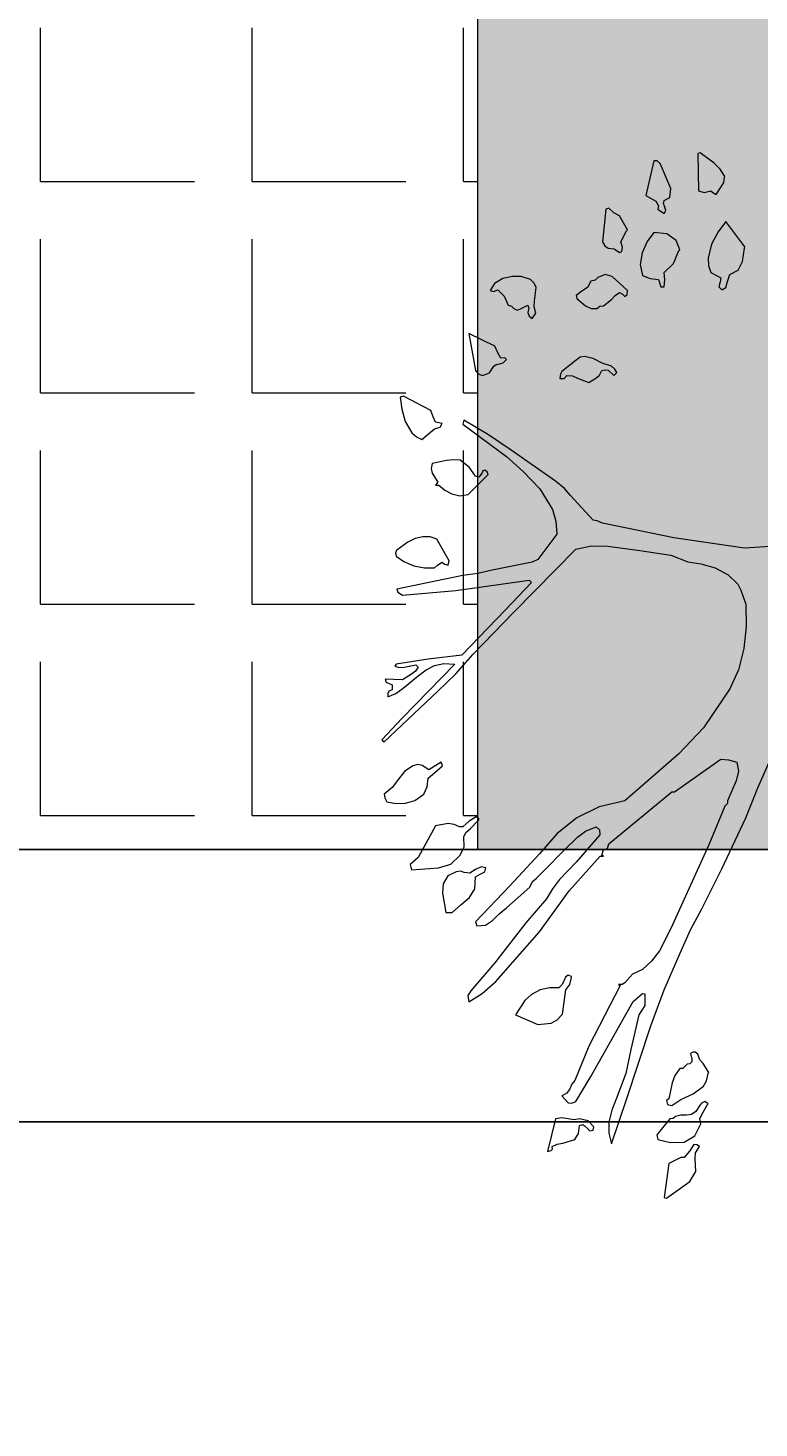
# Model space of a CAD drawing. Units: inches. Extents: x 84 to 1044, y -280 to 906.
# Tile 16 of 105: x 635 to 659, y -132 to -86. Entities that reach past the tile are written whole.
import ezdxf

# ---------------------------------------------------------------- set-up
doc = ezdxf.new("R2010")
doc.units = ezdxf.units.IN
for name, color, linetype, lineweight in [('A-ANNO-DIMS', 2, 'Continuous', 18), ('C-PROP', 7, 'Continuous', 25), ('L-HRDS', 32, 'Continuous', 18), ('L-PLNT', 114, 'Continuous', 15)]:
    doc.layers.add(name, color=color, linetype=linetype, lineweight=lineweight)
doc.layers.add('L-HRDS-PATT', color=23, linetype='Continuous', lineweight=9, true_color=0xc2877b)
doc.layers.add('L-PLNT-PATT', color=9, linetype='Continuous', lineweight=9, true_color=0xafd9aa)
doc.styles.get("Standard").update_dxf_attribs({"font": 'arial.ttf'})
doc.dimstyles.get("Standard").update_dxf_attribs({"dimtxt": 0.18, "dimasz": 0.18, "dimexe": 0.18, "dimexo": 0.0625, "dimgap": 0.09, "dimtad": 0, "dimtih": 1, "dimtoh": 1, "dimdec": 4, "dimzin": 0, "dimdsep": 46, "dimtxsty": 'Standard', "dimcen": 0.09, "dimadec": 0, "dimazin": 0, "dimtfac": 1, "dimtdec": 4, "dimtofl": 0, "dimtmove": 0, "dimatfit": 3, "dimfxl": 1, "dimtolj": 1, "dimtzin": 0, "dimarcsym": 0})

# ---------------------------------------------------------------- blocks, each defined once
blk = doc.blocks.new('A$C37E508DF')
for p, q in [((0.9686, 1.4334), (0.9875, 1.4476)), ((0.9875, 1.4476), (0.9905, 1.4467)), ((0.9905, 1.4467), (0.9896, 1.3966)), ((0.9605, 1.4257), (0.9686, 1.4334)), ((1.0269, 1.3996), (1.0411, 1.433)), ((1.0411, 1.433), (1.045, 1.4365)), ((1.045, 1.4365), (1.0497, 1.4369)), ((1.0497, 1.4369), (1.0604, 1.3901)), ((0.9545, 1.4159), (0.9605, 1.4257)), ((0.9549, 1.4146), (0.9545, 1.4159)), ((0.9558, 1.4077), (0.9549, 1.4146)), ((0.9592, 1.4017), (0.9558, 1.4077)), ((0.966, 1.3914), (0.9592, 1.4017)), ((0.9703, 1.3944), (0.966, 1.3914)), ((0.9733, 1.3966), (0.9703, 1.3944)), ((0.9819, 1.3944), (0.9733, 1.3966)), ((0.9896, 1.3966), (0.9819, 1.3944)), ((1.0282, 1.3876), (1.0269, 1.3996)), ((1.0604, 1.3901), (1.0471, 1.3824)), ((1.0359, 1.3833), (1.0282, 1.3876)), ((1.0334, 1.37), (1.0351, 1.376)), ((1.0351, 1.376), (1.0368, 1.3794)), ((1.0368, 1.3794), (1.0359, 1.3833)), ((1.0441, 1.3717), (1.0359, 1.3661)), ((1.0471, 1.3824), (1.0432, 1.3764)), ((1.0432, 1.3764), (1.0441, 1.3717)), ((1.1033, 1.367), (1.1097, 1.373)), ((1.1097, 1.373), (1.114, 1.3717)), ((1.114, 1.3717), (1.1183, 1.328)), ((0.9274, 1.3215), (0.9532, 1.3554)), ((0.9532, 1.3554), (0.9635, 1.3413)), ((1.0359, 1.3661), (1.0334, 1.37)), ((1.0848, 1.3443), (1.0955, 1.3631)), ((1.0955, 1.3631), (1.1033, 1.367)), ((0.9635, 1.3413), (0.9721, 1.325)), ((1.0197, 1.3297), (1.0321, 1.3387)), ((1.0321, 1.3387), (1.0497, 1.3404)), ((1.0497, 1.3404), (1.0587, 1.3284)), ((1.0861, 1.343), (1.0848, 1.3443)), ((1.0938, 1.328), (1.0861, 1.343)), ((0.9279, 1.3194), (0.9274, 1.3215)), ((0.9305, 1.3018), (0.9279, 1.3194)), ((0.9721, 1.325), (0.9768, 1.3061)), ((1.0149, 1.3172), (1.0171, 1.3232)), ((1.0162, 1.3164), (1.0149, 1.3172)), ((1.0231, 1.2988), (1.0162, 1.3164)), ((1.0171, 1.3232), (1.0197, 1.3297)), ((1.0587, 1.3284), (1.0651, 1.3134)), ((1.0917, 1.3207), (1.0938, 1.328)), ((1.0925, 1.3151), (1.0917, 1.3207)), ((1.0955, 1.3138), (1.0925, 1.3151)), ((1.1028, 1.3185), (1.0955, 1.3138)), ((1.111, 1.3194), (1.1028, 1.3185)), ((1.1153, 1.3228), (1.111, 1.3194)), ((1.1183, 1.328), (1.1153, 1.3228)), ((0.9365, 1.2902), (0.9305, 1.3018)), ((0.9763, 1.2962), (0.9733, 1.2868)), ((0.9768, 1.3061), (0.9763, 1.2962)), ((1.0359, 1.2868), (1.0231, 1.2988)), ((1.0677, 1.2975), (1.0647, 1.2829)), ((1.0651, 1.3134), (1.0677, 1.2975)), ((0.9476, 1.2842), (0.9365, 1.2902)), ((0.951, 1.2748), (0.9476, 1.2842)), ((0.9733, 1.2868), (0.9596, 1.2799)), ((0.9596, 1.2799), (0.9605, 1.2744)), ((1.0347, 1.2769), (1.0359, 1.2868)), ((1.0359, 1.2679), (1.0347, 1.2769)), ((1.0432, 1.2774), (1.0402, 1.2679)), ((1.0544, 1.2791), (1.0432, 1.2774)), ((1.0647, 1.2829), (1.0544, 1.2791)), ((1.0848, 1.2628), (1.1054, 1.2817)), ((1.1054, 1.2817), (1.1148, 1.2842)), ((1.1148, 1.2842), (1.1247, 1.2804)), ((1.1247, 1.2804), (1.1281, 1.2765)), ((1.21, 1.2726), (1.2147, 1.2774)), ((1.2147, 1.2774), (1.2276, 1.2817)), ((1.2276, 1.2817), (1.2392, 1.2817)), ((1.2392, 1.2817), (1.2521, 1.2787)), ((1.2521, 1.2787), (1.2632, 1.2722)), ((0.9532, 1.2666), (0.951, 1.2748)), ((0.9583, 1.2636), (0.9532, 1.2666)), ((0.9626, 1.2679), (0.9583, 1.2636)), ((0.9605, 1.2744), (0.9626, 1.2679)), ((1.0402, 1.2679), (1.0359, 1.2679)), ((1.0852, 1.2576), (1.0848, 1.2628)), ((1.0921, 1.2585), (1.0883, 1.2546)), ((1.0955, 1.2602), (1.0921, 1.2585)), ((1.1015, 1.2559), (1.0955, 1.2602)), ((1.1281, 1.2765), (1.1341, 1.2752)), ((1.1341, 1.2752), (1.1384, 1.2666)), ((1.1384, 1.2666), (1.1461, 1.2619)), ((1.1461, 1.2619), (1.1539, 1.2559)), ((1.2075, 1.2666), (1.21, 1.2726)), ((1.2096, 1.2491), (1.2075, 1.2666)), ((1.2585, 1.2636), (1.2503, 1.2551)), ((1.2645, 1.2615), (1.2585, 1.2636)), ((1.2632, 1.2722), (1.2692, 1.2628)), ((1.2692, 1.2628), (1.2645, 1.2615)), ((1.0883, 1.2546), (1.0852, 1.2576)), ((1.1063, 1.2508), (1.1015, 1.2559)), ((1.117, 1.2422), (1.1063, 1.2508)), ((1.1221, 1.2418), (1.117, 1.2422)), ((1.126, 1.2388), (1.1221, 1.2418)), ((1.141, 1.2422), (1.1337, 1.2388)), ((1.1526, 1.2521), (1.141, 1.2422)), ((1.1539, 1.2559), (1.1526, 1.2521)), ((1.2079, 1.2323), (1.21, 1.2409)), ((1.21, 1.2409), (1.2096, 1.2491)), ((1.2186, 1.2431), (1.2173, 1.2392)), ((1.2285, 1.2383), (1.2186, 1.2431)), ((1.2405, 1.2418), (1.2371, 1.2388)), ((1.2448, 1.2431), (1.2405, 1.2418)), ((1.2503, 1.2551), (1.2448, 1.2431)), ((1.1337, 1.2388), (1.126, 1.2388)), ((1.2126, 1.2251), (1.2079, 1.2323)), ((1.2169, 1.2285), (1.2126, 1.2251)), ((1.2186, 1.2332), (1.2169, 1.2285)), ((1.2173, 1.2392), (1.2186, 1.2332)), ((1.2328, 1.2366), (1.2285, 1.2383)), ((1.2371, 1.2388), (1.2328, 1.2366)), ((1.2628, 1.1882), (1.2975, 1.2053)), ((1.2975, 1.2053), (1.2885, 1.1556)), ((1.2589, 1.1792), (1.2628, 1.1882)), ((1.1063, 1.1612), (1.1187, 1.1655)), ((1.1187, 1.1655), (1.1307, 1.1714)), ((1.1307, 1.1714), (1.1423, 1.1744)), ((1.1423, 1.1744), (1.1483, 1.1732)), ((1.1483, 1.1732), (1.1539, 1.1693)), ((1.1539, 1.1693), (1.1727, 1.1543)), ((1.2469, 1.1702), (1.2495, 1.1723)), ((1.2478, 1.1693), (1.2469, 1.1702)), ((1.2516, 1.1659), (1.2478, 1.1693)), ((1.2495, 1.1723), (1.2546, 1.1719)), ((1.2563, 1.1646), (1.2516, 1.1659)), ((1.2546, 1.1719), (1.2589, 1.1792)), ((1.2611, 1.1637), (1.2563, 1.1646)), ((1.099, 1.153), (1.102, 1.1573)), ((1.1033, 1.1487), (1.099, 1.153)), ((1.102, 1.1573), (1.1063, 1.1612)), ((1.111, 1.156), (1.1033, 1.1487)), ((1.1153, 1.1564), (1.111, 1.156)), ((1.1191, 1.1556), (1.1153, 1.1564)), ((1.1226, 1.1492), (1.1191, 1.1556)), ((1.1273, 1.1453), (1.1226, 1.1492)), ((1.1586, 1.1483), (1.1517, 1.1453)), ((1.1663, 1.1487), (1.1586, 1.1483)), ((1.1697, 1.1449), (1.1663, 1.1487)), ((1.1727, 1.1543), (1.1749, 1.1504)), ((1.1749, 1.1504), (1.1757, 1.1449)), ((1.2641, 1.1612), (1.2611, 1.1637)), ((1.2701, 1.1522), (1.2641, 1.1612)), ((1.2791, 1.1487), (1.2701, 1.1522)), ((1.2851, 1.1509), (1.2791, 1.1487)), ((1.2885, 1.1556), (1.2851, 1.1509)), ((1.1367, 1.1393), (1.1273, 1.1453)), ((1.1517, 1.1453), (1.1367, 1.1393)), ((1.1757, 1.1449), (1.1697, 1.1449)), ((1.3485, 1.102), (1.385, 1.1209)), ((1.385, 1.1209), (1.3897, 1.1196)), ((1.3897, 1.1196), (1.3875, 1.1037)), ((1.3421, 1.0861), (1.3455, 1.0934)), ((1.3455, 1.0934), (1.3485, 1.102)), ((1.3875, 1.1037), (1.3828, 1.087)), ((1.3057, 1.0835), (1.2469, 1.0402)), ((1.2713, 1.0694), (1.3044, 1.0887)), ((1.3044, 1.0887), (1.3057, 1.0835)), ((1.3335, 1.0844), (1.3421, 1.0861)), ((1.3361, 1.0793), (1.3335, 1.0844)), ((1.3434, 1.0771), (1.3361, 1.0793)), ((1.349, 1.0728), (1.3434, 1.0771)), ((1.3605, 1.063), (1.349, 1.0728)), ((1.3738, 1.072), (1.3678, 1.0664)), ((1.3828, 1.087), (1.3738, 1.072)), ((1.2409, 1.0488), (1.2713, 1.0694)), ((1.3678, 1.0664), (1.3605, 1.063)), ((1.1813, 1.0072), (1.2409, 1.0488)), ((1.2469, 1.0402), (1.2246, 1.0201)), ((1.2971, 1.0257), (1.3091, 1.0351)), ((1.3091, 1.0351), (1.3185, 1.0355)), ((1.3185, 1.0355), (1.3275, 1.0347)), ((1.3275, 1.0347), (1.3468, 1.0308)), ((1.2246, 1.0201), (1.2023, 0.9969)), ((1.2718, 1.0162), (1.2731, 1.0197)), ((1.2984, 0.9892), (1.2718, 1.0162)), ((1.2731, 1.0197), (1.2761, 1.0218)), ((1.2761, 1.0218), (1.2786, 1.0209)), ((1.2786, 1.0209), (1.2799, 1.0184)), ((1.2799, 1.0184), (1.2842, 1.0124)), ((1.2885, 1.0136), (1.2971, 1.0257)), ((1.3468, 1.018), (1.3391, 1.0059)), ((1.3468, 1.0308), (1.3481, 1.0239)), ((1.3481, 1.0239), (1.3468, 1.018)), ((1.1612, 0.9879), (1.1693, 0.9974)), ((1.1693, 0.9974), (1.1813, 1.0072)), ((1.2023, 0.9969), (1.1852, 0.9691)), ((1.2842, 1.0124), (1.2885, 1.0136)), ((1.3297, 0.9952), (1.3202, 0.9901)), ((1.3378, 1.0016), (1.3297, 0.9952)), ((1.3421, 1.0016), (1.3378, 1.0016)), ((1.3391, 1.0059), (1.3421, 1.0016)), ((1.1311, 0.9549), (1.1612, 0.9879)), ((1.3095, 0.9875), (1.2984, 0.9892)), ((1.3202, 0.9901), (1.3095, 0.9875)), ((1.1852, 0.9691), (1.1809, 0.9532)), ((1.0227, 0.9309), (1.1183, 0.9506)), ((1.1183, 0.9506), (1.1256, 0.954)), ((1.1256, 0.954), (1.1311, 0.9549)), ((1.1809, 0.9532), (1.1796, 0.936)), ((0.9279, 0.9172), (1.0227, 0.9309)), ((1.1333, 0.9202), (1.1114, 0.9198)), ((1.1543, 0.9159), (1.1333, 0.9202)), ((1.1796, 0.936), (1.2049, 0.9022)), ((1.3241, 0.9), (1.3404, 0.9292)), ((1.3404, 0.9292), (1.3494, 0.9322)), ((1.3494, 0.9322), (1.3592, 0.9326)), ((1.3592, 0.9326), (1.3695, 0.93)), ((1.3695, 0.93), (1.3794, 0.9253)), ((1.3794, 0.9253), (1.394, 0.9146)), ((0.8936, 0.9193), (0.9279, 0.9172)), ((1.0269, 0.9077), (1.0042, 0.8987)), ((1.0685, 0.9142), (1.0269, 0.9077)), ((1.1114, 0.9198), (1.0685, 0.9142)), ((1.2371, 0.8314), (1.1543, 0.9159)), ((1.2049, 0.9022), (1.2126, 0.8983)), ((1.3948, 0.9065), (1.3846, 0.8992)), ((1.394, 0.9146), (1.3957, 0.9112)), ((1.3957, 0.9112), (1.3948, 0.9065)), ((0.9673, 0.8906), (0.9498, 0.8816)), ((0.9866, 0.8962), (0.9673, 0.8906)), ((1.0042, 0.8987), (0.9866, 0.8962)), ((1.2126, 0.8983), (1.2662, 0.8876)), ((1.2662, 0.8876), (1.2855, 0.8833)), ((1.2855, 0.8833), (1.3057, 0.8807)), ((1.3254, 0.8944), (1.3241, 0.9)), ((1.3301, 0.8957), (1.3254, 0.8944)), ((1.3335, 0.8983), (1.3301, 0.8957)), ((1.3395, 0.8944), (1.3335, 0.8983)), ((1.3434, 0.8906), (1.3395, 0.8944)), ((1.3571, 0.8906), (1.3434, 0.8906)), ((1.3713, 0.8936), (1.3571, 0.8906)), ((1.3846, 0.8992), (1.3713, 0.8936)), ((0.9369, 0.8687), (0.933, 0.861)), ((0.9498, 0.8816), (0.9369, 0.8687)), ((1.2169, 0.8743), (1.2135, 0.8713)), ((1.2135, 0.8713), (1.2491, 0.834)), ((1.3151, 0.8606), (1.2169, 0.8743)), ((1.3057, 0.8807), (1.394, 0.8623)), ((0.9296, 0.852), (0.9262, 0.8421)), ((0.933, 0.861), (0.9296, 0.852)), ((1.3863, 0.8541), (1.3151, 0.8606)), ((1.3927, 0.8584), (1.3863, 0.8541)), ((1.394, 0.8623), (1.3927, 0.8584)), ((0.9262, 0.8421), (0.9257, 0.8121)), ((1.2919, 0.7752), (1.2371, 0.8314)), ((1.2491, 0.834), (1.3069, 0.7735)), ((0.9257, 0.8121), (0.9287, 0.7825)), ((0.9287, 0.7825), (0.936, 0.7542)), ((1.3151, 0.7487), (1.2919, 0.7752)), ((1.3069, 0.7735), (1.352, 0.7684)), ((0.936, 0.7542), (0.9476, 0.7285)), ((1.3309, 0.7624), (1.3164, 0.7615)), ((1.3164, 0.7615), (1.3871, 0.6891)), ((1.3434, 0.7598), (1.3309, 0.7624)), ((1.355, 0.7538), (1.3434, 0.7598)), ((1.352, 0.7684), (1.3948, 0.7615)), ((1.3653, 0.7461), (1.355, 0.7538)), ((1.3687, 0.7607), (1.3657, 0.7577)), ((1.3657, 0.7577), (1.3691, 0.7521)), ((1.3841, 0.7577), (1.3687, 0.7607)), ((1.3691, 0.7521), (1.3743, 0.7482)), ((1.3914, 0.7572), (1.3841, 0.7577)), ((1.397, 0.759), (1.3914, 0.7572)), ((1.3948, 0.7615), (1.397, 0.759)), ((1.3391, 0.7255), (1.3151, 0.7487)), ((1.3854, 0.7294), (1.3653, 0.7461)), ((1.3743, 0.7482), (1.3863, 0.7405)), ((1.3863, 0.7405), (1.4099, 0.7414)), ((1.4086, 0.7375), (1.4004, 0.7337)), ((1.4004, 0.7337), (1.4004, 0.7272)), ((1.4099, 0.7414), (1.4086, 0.7375)), ((0.9476, 0.7285), (0.9828, 0.6762)), ((1.4116, 0.6569), (1.3391, 0.7255)), ((1.3953, 0.7221), (1.3854, 0.7294)), ((1.4064, 0.7178), (1.3953, 0.7221)), ((1.4004, 0.7272), (1.4047, 0.7255)), ((1.4047, 0.7255), (1.406, 0.7221)), ((1.406, 0.7221), (1.4064, 0.7178)), ((0.9828, 0.6762), (1.0162, 0.6415)), ((1.3871, 0.6891), (1.4141, 0.6599)), ((1.4141, 0.6599), (1.4116, 0.6569)), ((1.0162, 0.6415), (1.0574, 0.605)), ((0.9103, 0.5956), (0.8932, 0.6342)), ((0.9382, 0.6303), (0.936, 0.6179)), ((0.9493, 0.6333), (0.9382, 0.6303)), ((0.9596, 0.6342), (0.9493, 0.6333)), ((1.0218, 0.5904), (0.9596, 0.6342)), ((1.3327, 0.6252), (1.3348, 0.6303)), ((1.343, 0.6162), (1.3327, 0.6252)), ((1.3348, 0.6303), (1.3511, 0.62)), ((1.3511, 0.62), (1.3601, 0.6256)), ((1.3601, 0.6256), (1.3661, 0.6269)), ((1.3661, 0.6269), (1.3725, 0.6252)), ((1.3725, 0.6252), (1.3837, 0.6175)), ((0.936, 0.6179), (0.939, 0.605)), ((0.939, 0.605), (0.9506, 0.5784)), ((1.0574, 0.605), (1.0883, 0.5784)), ((1.352, 0.6089), (1.343, 0.6162)), ((1.3533, 0.5969), (1.352, 0.6089)), ((1.3837, 0.6175), (1.3918, 0.6072)), ((1.3918, 0.6072), (1.4004, 0.5964)), ((0.9262, 0.5557), (0.9103, 0.5956)), ((1.0256, 0.5904), (1.0218, 0.5904)), ((1.1097, 0.5205), (1.0256, 0.5904)), ((1.358, 0.5874), (1.3533, 0.5969)), ((1.37, 0.5789), (1.358, 0.5874)), ((1.4004, 0.5964), (1.4111, 0.5874)), ((1.4103, 0.5823), (1.4077, 0.5771)), ((1.4111, 0.5874), (1.4103, 0.5823)), ((0.9506, 0.5784), (0.951, 0.5746)), ((0.951, 0.5746), (0.9545, 0.5711)), ((0.9545, 0.5711), (0.9759, 0.5193)), ((1.0883, 0.5784), (1.123, 0.5703)), ((1.123, 0.5703), (1.1526, 0.5557)), ((1.3824, 0.575), (1.37, 0.5789)), ((1.3953, 0.5746), (1.3824, 0.575)), ((1.4077, 0.5771), (1.3953, 0.5746)), ((0.9583, 0.4871), (0.9262, 0.5557)), ((1.1526, 0.5557), (1.1792, 0.5347)), ((1.2842, 0.554), (1.2855, 0.5557)), ((1.2842, 0.5527), (1.2842, 0.554)), ((1.2958, 0.5407), (1.2842, 0.5527)), ((1.2855, 0.5557), (1.2876, 0.557)), ((1.2876, 0.557), (1.2971, 0.551)), ((1.2971, 0.551), (1.3057, 0.5433)), ((1.3099, 0.5433), (1.3172, 0.5467)), ((1.3172, 0.5467), (1.3254, 0.548)), ((1.3254, 0.548), (1.3421, 0.5446)), ((1.3421, 0.5446), (1.3657, 0.5021)), ((1.1226, 0.5394), (1.1221, 0.5325)), ((1.1221, 0.5325), (1.1539, 0.4961)), ((1.1268, 0.5433), (1.1226, 0.5394)), ((1.141, 0.5377), (1.1268, 0.5433)), ((1.1521, 0.5296), (1.141, 0.5377)), ((1.1706, 0.5111), (1.1521, 0.5296)), ((1.1792, 0.5347), (1.2027, 0.5072)), ((1.3014, 0.536), (1.2958, 0.5407)), ((1.3044, 0.53), (1.3014, 0.536)), ((1.3039, 0.5167), (1.3044, 0.53)), ((1.3057, 0.5433), (1.3099, 0.5433)), ((0.9759, 0.5193), (1.0269, 0.4069)), ((1.1118, 0.5145), (1.1097, 0.5205)), ((1.117, 0.5124), (1.1118, 0.5145)), ((1.1191, 0.5055), (1.117, 0.5124)), ((1.1955, 0.4858), (1.1706, 0.5111)), ((1.2027, 0.5072), (1.2426, 0.4644)), ((1.3091, 0.5055), (1.3039, 0.5167)), ((1.117, 0.5042), (1.1191, 0.5055)), ((1.1217, 0.5042), (1.117, 0.5042)), ((1.1633, 0.4575), (1.1217, 0.5042)), ((1.1539, 0.4961), (1.1762, 0.4729)), ((1.2748, 0.4884), (1.2812, 0.4897)), ((1.2761, 0.4832), (1.2748, 0.4884)), ((1.2812, 0.4897), (1.2885, 0.4862)), ((1.3215, 0.4935), (1.3091, 0.5055)), ((1.3382, 0.4884), (1.3215, 0.4935)), ((1.3743, 0.4858), (1.3382, 0.4884)), ((1.3657, 0.5021), (1.3764, 0.4927)), ((1.3764, 0.4927), (1.3743, 0.4858)), ((0.9853, 0.4335), (0.9583, 0.4871)), ((1.1762, 0.4729), (1.1856, 0.4605)), ((1.207, 0.4747), (1.1955, 0.4858)), ((1.2122, 0.47), (1.207, 0.4747)), ((1.2156, 0.4627), (1.2122, 0.47)), ((1.2825, 0.4798), (1.2761, 0.4832)), ((1.2885, 0.4764), (1.2825, 0.4798)), ((1.2885, 0.4862), (1.2962, 0.4815)), ((1.2894, 0.4601), (1.2885, 0.4764)), ((1.2962, 0.4815), (1.3039, 0.482)), ((1.3039, 0.482), (1.3087, 0.4841)), ((1.3087, 0.4841), (1.3147, 0.4832)), ((1.3147, 0.4832), (1.3258, 0.4777)), ((1.3258, 0.4777), (1.3318, 0.4669)), ((1.2027, 0.4026), (1.1633, 0.4575)), ((1.1856, 0.4605), (1.1933, 0.4468)), ((1.2469, 0.4348), (1.2156, 0.4627)), ((1.2426, 0.4644), (1.2885, 0.4159)), ((1.2967, 0.4485), (1.2894, 0.4601)), ((1.3331, 0.4545), (1.3284, 0.4284)), ((1.3318, 0.4669), (1.3331, 0.4545)), ((1.0003, 0.4052), (0.9853, 0.4335)), ((1.1933, 0.4468), (1.2212, 0.4146)), ((1.2568, 0.4266), (1.2469, 0.4348)), ((1.3082, 0.4386), (1.2967, 0.4485)), ((1.3198, 0.4284), (1.3082, 0.4386)), ((1.2212, 0.4146), (1.2628, 0.361)), ((1.2658, 0.4176), (1.2568, 0.4266)), ((1.2752, 0.4116), (1.2658, 0.4176)), ((1.2885, 0.4159), (1.2868, 0.4108)), ((1.3284, 0.4284), (1.3198, 0.4284)), ((1.0145, 0.373), (1.0003, 0.4052)), ((1.0269, 0.4069), (1.0419, 0.3769)), ((1.2289, 0.373), (1.2027, 0.4026)), ((1.2868, 0.4108), (1.2752, 0.4116)), ((1.0419, 0.3769), (1.0527, 0.3632)), ((1.0359, 0.3246), (1.0145, 0.373)), ((1.0527, 0.3632), (1.0647, 0.352)), ((1.2615, 0.3362), (1.2289, 0.373)), ((1.2628, 0.361), (1.2949, 0.3233)), ((1.0647, 0.352), (1.078, 0.346)), ((1.078, 0.346), (1.0883, 0.334)), ((1.1599, 0.3426), (1.1646, 0.3447)), ((1.1599, 0.3413), (1.1599, 0.3426)), ((1.162, 0.3319), (1.1599, 0.3413)), ((1.1646, 0.3447), (1.168, 0.3417)), ((1.168, 0.3417), (1.1702, 0.3366)), ((1.0535, 0.2766), (1.0359, 0.3246)), ((1.0647, 0.3199), (1.0617, 0.3194)), ((1.0617, 0.3194), (1.0617, 0.304)), ((1.0711, 0.3147), (1.0647, 0.3199)), ((1.0883, 0.334), (1.0921, 0.3319)), ((1.0921, 0.3319), (1.0968, 0.3319)), ((1.0968, 0.3319), (1.0947, 0.3306)), ((1.0947, 0.3306), (1.1367, 0.2491)), ((1.1676, 0.325), (1.162, 0.3319)), ((1.1719, 0.292), (1.1676, 0.325)), ((1.1702, 0.3366), (1.1727, 0.3314)), ((1.1727, 0.3314), (1.177, 0.3276)), ((1.177, 0.3276), (1.1895, 0.3276)), ((1.1895, 0.3276), (1.2019, 0.3246)), ((1.2019, 0.3246), (1.2135, 0.3186)), ((1.2795, 0.3199), (1.2615, 0.3362)), ((1.2975, 0.3087), (1.2795, 0.3199)), ((1.2949, 0.3233), (1.2988, 0.3173)), ((1.0617, 0.304), (1.0698, 0.2911)), ((1.0775, 0.3092), (1.0711, 0.3147)), ((1.1341, 0.2084), (1.0775, 0.3092)), ((1.2135, 0.3186), (1.2225, 0.3104)), ((1.2225, 0.3104), (1.2349, 0.2911)), ((1.2988, 0.3173), (1.2975, 0.3087)), ((1.0698, 0.2911), (1.0805, 0.2448)), ((1.1792, 0.2847), (1.1719, 0.292)), ((1.1873, 0.28), (1.1792, 0.2847)), ((1.2349, 0.2911), (1.2049, 0.2783)), ((1.0861, 0.1775), (1.0535, 0.2766)), ((1.2049, 0.2783), (1.1873, 0.28)), ((1.0805, 0.2448), (1.087, 0.2127)), ((1.1367, 0.2491), (1.1556, 0.2032)), ((0.9759, 0.214), (0.9836, 0.226)), ((0.9836, 0.226), (0.9879, 0.2311)), ((0.9879, 0.2311), (0.9905, 0.2384)), ((0.9905, 0.2384), (0.9943, 0.241)), ((0.9943, 0.241), (0.9973, 0.2414)), ((0.9973, 0.2414), (1.0003, 0.2393)), ((1.0003, 0.2393), (0.9986, 0.232)), ((0.9986, 0.232), (0.9986, 0.2281)), ((0.9986, 0.2281), (1.0012, 0.2255)), ((1.0012, 0.2255), (1.0051, 0.2251)), ((0.9768, 0.2127), (0.9759, 0.214)), ((0.9789, 0.2028), (0.9768, 0.2127)), ((1.0051, 0.2251), (1.0076, 0.2225)), ((1.0076, 0.2225), (1.0106, 0.2195)), ((1.0106, 0.2195), (1.0149, 0.2191)), ((1.0149, 0.2191), (1.0214, 0.2101)), ((1.0214, 0.2101), (1.0252, 0.2002)), ((1.087, 0.2127), (1.0998, 0.1797)), ((1.1543, 0.1749), (1.1341, 0.2084)), ((0.9832, 0.1955), (0.9789, 0.2028)), ((0.9969, 0.1852), (0.9832, 0.1955)), ((1.0252, 0.2002), (1.0295, 0.1788)), ((1.1556, 0.2032), (1.1594, 0.1985)), ((1.1594, 0.1985), (1.1624, 0.1921)), ((1.1624, 0.1921), (1.1663, 0.1861)), ((0.9768, 0.1719), (0.9811, 0.1749)), ((0.9776, 0.1711), (0.9768, 0.1719)), ((0.9853, 0.1578), (0.9776, 0.1711)), ((0.9811, 0.1749), (0.9858, 0.1728)), ((0.9858, 0.1728), (0.9884, 0.1694)), ((0.9884, 0.1694), (0.9931, 0.1616)), ((1.0132, 0.1779), (0.9969, 0.1852)), ((1.0256, 0.1698), (1.0132, 0.1779)), ((1.0312, 0.1711), (1.0256, 0.1698)), ((1.0295, 0.1788), (1.0325, 0.1762)), ((1.0325, 0.1762), (1.0312, 0.1711)), ((1.1063, 0.1183), (1.0861, 0.1775)), ((1.0998, 0.1797), (1.1058, 0.1634)), ((1.1594, 0.1728), (1.1543, 0.1749)), ((1.1646, 0.1732), (1.1594, 0.1728)), ((1.1727, 0.1827), (1.1646, 0.1732)), ((1.1663, 0.1861), (1.1727, 0.1827)), ((0.9879, 0.1518), (0.9853, 0.1578)), ((0.9866, 0.1453), (0.9879, 0.1518)), ((0.9931, 0.1616), (0.9991, 0.1574)), ((0.9991, 0.1574), (1.0059, 0.1565)), ((1.0059, 0.1565), (1.0132, 0.1565)), ((1.0132, 0.1565), (1.0205, 0.1548)), ((1.0205, 0.1548), (1.0235, 0.1522)), ((1.0235, 0.1522), (1.0282, 0.1518)), ((1.0282, 0.1518), (1.0454, 0.1303)), ((1.1058, 0.1634), (1.1097, 0.1475)), ((1.1376, 0.1492), (1.1491, 0.1518)), ((1.1491, 0.1518), (1.1564, 0.1505)), ((1.1564, 0.1505), (1.1642, 0.1518)), ((1.1642, 0.1518), (1.1727, 0.1531)), ((1.1727, 0.1531), (1.1813, 0.1518)), ((1.1813, 0.1518), (1.192, 0.108)), ((0.9948, 0.1291), (0.9866, 0.1453)), ((1.1101, 0.1325), (1.1063, 0.1183)), ((1.1097, 0.1475), (1.1101, 0.1325)), ((1.1298, 0.1411), (1.1376, 0.1492)), ((1.1311, 0.1364), (1.1298, 0.1411)), ((1.1354, 0.1359), (1.1311, 0.1364)), ((1.1384, 0.1389), (1.1354, 0.1359)), ((1.1423, 0.1423), (1.1384, 0.1389)), ((1.1449, 0.1441), (1.1423, 0.1423)), ((1.1491, 0.1428), (1.1449, 0.1441)), ((1.1504, 0.132), (1.1491, 0.1428)), ((1.1556, 0.1239), (1.1504, 0.132)), ((0.9884, 0.1149), (0.9918, 0.117)), ((0.9935, 0.1063), (0.9884, 0.1149)), ((0.9918, 0.117), (0.9961, 0.1175)), ((1.0089, 0.1205), (0.9948, 0.1291)), ((0.9961, 0.1175), (1.0016, 0.1085)), ((1.0274, 0.12), (1.0089, 0.1205)), ((1.0441, 0.1239), (1.0274, 0.12)), ((1.0454, 0.1303), (1.0441, 0.1239)), ((1.1714, 0.1192), (1.1556, 0.1239)), ((1.1792, 0.1179), (1.1714, 0.1192)), ((1.186, 0.1145), (1.1792, 0.1179)), ((1.1856, 0.111), (1.186, 0.1145)), ((0.9931, 0.081), (0.9943, 0.0982)), ((0.9943, 0.0982), (0.9935, 0.1063)), ((1.0016, 0.1085), (1.0089, 0.0999)), ((1.0089, 0.0999), (1.0132, 0.0999)), ((1.0132, 0.0999), (1.0295, 0.0917)), ((1.1873, 0.1093), (1.1856, 0.111)), ((1.192, 0.108), (1.1873, 0.1093)), ((1.0012, 0.0677), (0.9931, 0.081)), ((1.0295, 0.0917), (1.0359, 0.0463)), ((1.0325, 0.0454), (1.0012, 0.0677)), ((1.0359, 0.0463), (1.0325, 0.0454))]:
    blk.add_line(p, q)
blk = doc.blocks.new('*D60')
at = {"layer": 'A-ANNO-DIMS', "color": 0, "lineweight": -2, "transparency": 16777216}
for p, q in [((134.179, -121.942), (134.179, -180.64)), ((992.074, -121.942), (992.074, -180.64)), ((134.359, -180.46), (562.733, -180.46)), ((991.894, -180.46), (563.521, -180.46))]:
    blk.add_line(p, q, dxfattribs=at)
at = {"layer": 'A-ANNO-DIMS', "color": 0, "transparency": 16777216}
for points in [[(134.359, -180.43), (134.359, -180.49), (134.179, -180.46)], [(991.894, -180.43), (991.894, -180.49), (992.074, -180.46)]]:
    blk.add_solid(points, dxfattribs=at)
at = {"layer": 'Defpoints', "color": 0, "transparency": 16777216}
for p in [(134.179, -121.88), (992.074, -121.88), (992.074, -180.46)]:
    blk.add_point(p, dxfattribs=at)
at = {"layer": 'A-ANNO-DIMS', "color": 0, "transparency": 16777216, "insert": (563.127, -180.46), "char_height": 0.18, "attachment_point": 5}
blk.add_mtext('\\A1;857.9', dxfattribs=at)

msp = doc.modelspace()

# ---------------------------------------------------------------- hatches: boundary and pattern name
at = {"layer": 'L-HRDS-PATT', "transparency": 33554567}
h = msp.add_hatch(dxfattribs=at)
h.set_pattern_fill('ANGLE', color=256)
h.set_pattern_definition([(0, (0, 0), (0, 6.985), [5.08, -1.905]), (90, (0, 0), (-6.985, 4e-16), [5.08, -1.905])])
h.paths.add_polyline_path([(650.074, 31.12), (504.574, 31.12), (504.574, -112.88), (504.574, -121.88), (624.574, -121.88), (624.574, -112.88), (650.074, -112.88)])
at = {"layer": 'L-PLNT-PATT', "transparency": 33554597}
h = msp.add_hatch(color=256, dxfattribs=at)
h.dxf.hatch_style = 1
h.paths.add_polyline_path([(791.074, 31.12), (791.074, 91.12), (743.074, 91.12), (674.074, 91.12), (674.074, 31.12), (650.074, 31.12), (650.074, -112.88), (983.074, -112.88), (983.074, -64.88), (791.074, -64.88)])

# ---------------------------------------------------------------- linework, layer by layer
at = {"layer": 'C-PROP'}
for points in [[(143.179, -121.88), (134.179, -121.88), (134.179, 856.12), (992.074, 856.12), (992.074, -121.88), (624.574, -121.88)], [(143.179, -112.88), (143.179, 847.12), (983.074, 847.12), (983.074, -112.88), (624.574, -112.88)]]:
    msp.add_lwpolyline(points, dxfattribs=at)
at = {"layer": 'L-HRDS'}
msp.add_line((650.074, 31.12), (650.074, -112.88), dxfattribs=at)

# ---------------------------------------------------------------- block references
at = {"layer": 'L-PLNT', "xscale": -24.64361536662419, "yscale": 24.64361536662419, "zscale": 24.64361536662419}
msp.add_blockref('A$C37E508DF', (681.765, -125.52), dxfattribs=at)

# ---------------------------------------------------------------- dimensions: what is measured, and where the dimension line sits
at = {"layer": 'A-ANNO-DIMS'}
dim = msp.add_linear_dim(base=(992.074, -180.46), p1=(134.179, -121.88), p2=(992.074, -121.88), dimstyle='Standard', override={"dimdec": 1, "dimlfac": 1, "dimrnd": 0, "dimzin": 0, "dimdsep": 46, "dimlunit": 2}, dxfattribs=at)
dim.commit()
dim.dimension.update_dxf_attribs({"geometry": '*D60', "text_midpoint": (563.127, -180.46)})

doc.saveas('drawing.dxf')
